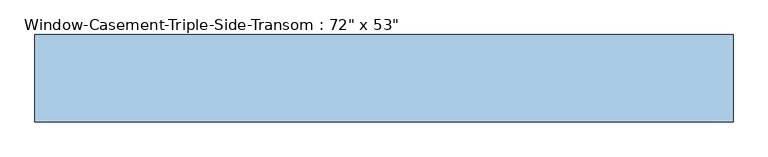
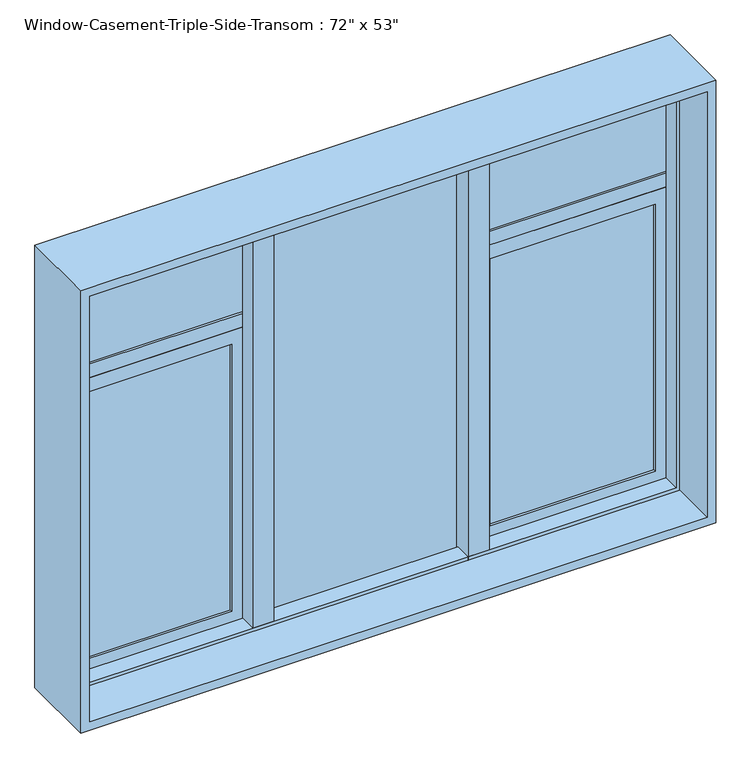
"""IFC4 building model written with IfcOpenShell, lengths in millimetres: window geometry."""

from ifc_helpers import new_model, si_unit, frame, origin, place, context, project, spatial, polyline, outline, extrude, faceted_brep, source, transform, mapped, element, save


def window_dd70d674(model_context):
    return source(origin(), model_context, "Body", "SolidModel", [
        faceted_brep([(-889.0, 73.025, 2235.2), (-889.0, 114.3, 2235.2), (889.0, 114.3, 2235.2), (889.0, 73.025, 2235.2), (-878.8796875, 22.225, 2225.0796875), (-878.8796875, 73.025, 2225.0796875), (878.8796875, 73.025, 2225.0796875), (878.8796875, 22.225, 2225.0796875), (-889.0, -114.3, 2235.2), (-889.0, 22.225, 2235.2), (889.0, 22.225, 2235.2), (889.0, -114.3, 2235.2), (-914.4, 114.3, 2260.6), (-914.4, -114.3, 2260.6), (914.4, -114.3, 2260.6), (914.4, 114.3, 2260.6), (889.0, 114.3, 939.8), (889.0, 73.025, 939.8), (878.8796875, 73.025, 949.9203125), (878.8796875, 22.225, 949.9203125), (889.0, 22.225, 939.8), (889.0, -114.3, 939.8), (914.4, -114.3, 914.4), (914.4, 114.3, 914.4), (-889.0, 114.3, 939.8), (-889.0, 73.025, 939.8), (-878.8796875, 73.025, 949.9203125), (-878.8796875, 22.225, 949.9203125), (-889.0, 22.225, 939.8), (-889.0, -114.3, 939.8), (-914.4, -114.3, 914.4), (-914.4, 114.3, 914.4)], [[[0, 1, 2, 3]], [[4, 5, 6, 7]], [[8, 9, 10, 11]], [[12, 13, 14, 15]], [[3, 2, 16, 17]], [[7, 6, 18, 19]], [[11, 10, 20, 21]], [[15, 14, 22, 23]], [[17, 16, 24, 25]], [[19, 18, 26, 27]], [[21, 20, 28, 29]], [[23, 22, 30, 31]], [[25, 24, 1, 0]], [[3, 17, 25, 0], [5, 26, 18, 6]], [[27, 26, 5, 4]], [[9, 28, 20, 10], [7, 19, 27, 4]], [[29, 28, 9, 8]], [[13, 30, 22, 14], [11, 21, 29, 8]], [[31, 30, 13, 12]], [[15, 23, 31, 12], [1, 24, 16, 2]]]),
        extrude(outline(polyline([(-279.4, 111.125), (-279.4, 22.225), (-340.3203125, 22.225), (-340.3203125, 73.025), (-330.2, 73.025), (-330.2, 111.125), (-279.4, 111.125)])), frame((0.0, 0.0, 939.8), z_axis=(0.0, 0.0, 1.0), x_axis=(1.0, 0.0, 0.0)), (0.0, 0.0, 1.0), 1295.4),
        extrude(outline(polyline([(330.2, 111.125), (330.2, 73.025), (340.3203125, 73.025), (340.3203125, 22.225), (279.4, 22.225), (279.4, 111.125), (330.2, 111.125)])), frame((0.0, 0.0, 939.8), z_axis=(0.0, 0.0, 1.0), x_axis=(1.0, 0.0, 0.0)), (0.0, 0.0, 1.0), 1295.4),
        extrude(outline(polyline([(1835.8048438, 330.2), (939.8, 330.2), (939.8, 889.0), (1835.8048438, 889.0), (1835.8048438, 330.2)]), holes=[polyline([(1793.9345313, 847.1296875), (981.6703125, 847.1296875), (981.6703125, 372.0703125), (1793.9345313, 372.0703125), (1793.9345313, 847.1296875)])]), frame((0.0, 73.025, 0.0), z_axis=(0.0, 1.0, 0.0), x_axis=(0.0, 0.0, 1.0)), (0.0, 0.0, 1.0), 31.75),
        extrude(outline(polyline([(1835.8048438, -889.0), (939.8, -889.0), (939.8, -330.2), (1835.8048438, -330.2), (1835.8048438, -889.0)]), holes=[polyline([(1793.9345313, -372.0703125), (981.6703125, -372.0703125), (981.6703125, -847.1296875), (1793.9345313, -847.1296875), (1793.9345313, -372.0703125)])]), frame((0.0, 73.025, 0.0), z_axis=(0.0, 1.0, 0.0), x_axis=(0.0, 0.0, 1.0)), (0.0, 0.0, 1.0), 31.75),
        extrude(outline(polyline([(-372.0703125, 98.425), (-372.0703125, 92.075), (-847.1296875, 92.075), (-847.1296875, 98.425), (-372.0703125, 98.425)])), frame((0.0, 0.0, 981.6703125), z_axis=(0.0, 0.0, 1.0), x_axis=(1.0, 0.0, 0.0)), (0.0, 0.0, 1.0), 812.2642188),
        extrude(outline(polyline([(-372.0703125, 85.725), (-372.0703125, 79.375), (-847.1296875, 79.375), (-847.1296875, 85.725), (-372.0703125, 85.725)])), frame((0.0, 0.0, 981.6703125), z_axis=(0.0, 0.0, 1.0), x_axis=(1.0, 0.0, 0.0)), (0.0, 0.0, 1.0), 812.2642188),
        extrude(outline(polyline([(847.1296875, 98.425), (847.1296875, 92.075), (372.0703125, 92.075), (372.0703125, 98.425), (847.1296875, 98.425)])), frame((0.0, 0.0, 981.6703125), z_axis=(0.0, 0.0, 1.0), x_axis=(1.0, 0.0, 0.0)), (0.0, 0.0, 1.0), 812.2642188),
        extrude(outline(polyline([(847.1296875, 85.725), (847.1296875, 79.375), (372.0703125, 79.375), (372.0703125, 85.725), (847.1296875, 85.725)])), frame((0.0, 0.0, 981.6703125), z_axis=(0.0, 0.0, 1.0), x_axis=(1.0, 0.0, 0.0)), (0.0, 0.0, 1.0), 812.2642188),
        extrude(outline(polyline([(889.0, 104.775), (889.0, 73.025), (330.2, 73.025), (330.2, 104.775), (889.0, 104.775)])), frame((0.0, 0.0, 1835.8048438), z_axis=(0.0, 0.0, 1.0), x_axis=(1.0, 0.0, 0.0)), (0.0, 0.0, 1.0), 41.8703125),
        extrude(outline(polyline([(279.4, 98.425), (279.4, 92.075), (-279.4, 92.075), (-279.4, 98.425), (279.4, 98.425)])), frame((0.0, 0.0, 939.8), z_axis=(0.0, 0.0, 1.0), x_axis=(1.0, 0.0, 0.0)), (0.0, 0.0, 1.0), 1295.4),
        extrude(outline(polyline([(279.4, 85.725), (279.4, 79.375), (-279.4, 79.375), (-279.4, 85.725), (279.4, 85.725)])), frame((0.0, 0.0, 939.8), z_axis=(0.0, 0.0, 1.0), x_axis=(1.0, 0.0, 0.0)), (0.0, 0.0, 1.0), 1295.4),
        extrude(outline(polyline([(-330.2, 104.775), (-330.2, 73.025), (-889.0, 73.025), (-889.0, 104.775), (-330.2, 104.775)])), frame((0.0, 0.0, 1835.8048438), z_axis=(0.0, 0.0, 1.0), x_axis=(1.0, 0.0, 0.0)), (0.0, 0.0, 1.0), 41.8703125),
        extrude(outline(polyline([(-330.2, 98.425), (-330.2, 92.075), (-889.0, 92.075), (-889.0, 98.425), (-330.2, 98.425)])), frame((0.0, 0.0, 1877.6751562), z_axis=(0.0, 0.0, 1.0), x_axis=(1.0, 0.0, 0.0)), (0.0, 0.0, 1.0), 357.5248438),
        extrude(outline(polyline([(-330.2, 85.725), (-330.2, 79.375), (-889.0, 79.375), (-889.0, 85.725), (-330.2, 85.725)])), frame((0.0, 0.0, 1877.6751562), z_axis=(0.0, 0.0, 1.0), x_axis=(1.0, 0.0, 0.0)), (0.0, 0.0, 1.0), 357.5248438),
        extrude(outline(polyline([(889.0, 98.425), (889.0, 92.075), (330.2, 92.075), (330.2, 98.425), (889.0, 98.425)])), frame((0.0, 0.0, 1877.6751562), z_axis=(0.0, 0.0, 1.0), x_axis=(1.0, 0.0, 0.0)), (0.0, 0.0, 1.0), 357.5248438),
        extrude(outline(polyline([(889.0, 85.725), (889.0, 79.375), (330.2, 79.375), (330.2, 85.725), (889.0, 85.725)])), frame((0.0, 0.0, 1877.6751562), z_axis=(0.0, 0.0, 1.0), x_axis=(1.0, 0.0, 0.0)), (0.0, 0.0, 1.0), 357.5248438),
    ])


if __name__ == "__main__":
    model = new_model("IFC4")
    model_context = context("Model", 3, world=origin())
    ifc_project = project(units=[si_unit("LENGTHUNIT", "METRE", prefix="MILLI")], contexts=[model_context])
    site = spatial("IfcSite", under=ifc_project)
    building = spatial("IfcBuilding", under=site)
    placement = place(None, origin())
    window_shape = window_dd70d674(model_context)
    element("IfcWindow", 1, ObjectType="Window-Casement-Triple-Side-Transom : 72\" x 53\"", at=placement, inside=building, context=model_context, shape_type="MappedRepresentation", body=[
        mapped(window_shape, transform((0.0, 0.0, 0.0), x_axis=(1.0, 0.0, 0.0), y_axis=(0.0, 1.0, 0.0), z_axis=(0.0, 0.0, 1.0))),
    ])
    save(model, "model.ifc")

# Revit data of these elements
# Type "Window-Casement-Triple-Side-Transom : 72\" x 53\""
#   Type Mark = "19"
#   Fire Rating = "0.5h"
#   Analytic Construction = "Double glazing - domestic"
#   Window Width = 2' - 0"
#   Window Inset [instance default] = 0' - 0 5/8"
#   Wall Thickness [instance default] = 0' - 6"
#   Visual Light Transmittance = 0.81
#   Transom Height Ratio = 0.3
#   Thermal Resistance (R) = 1.8146 (h·ft²·°F)/BTU
#   Solar Heat Gain Coefficient = 0.76
#   Rough Width = 6' - 0 1/2"
#   Rough Height = 4' - 5 1/2"
#   Open Window Height = 3' - 1.1"
#   Heat Transfer Coefficient (U) = 0.5511 BTU/(h·ft²·°F)
#   Height = 4' - 5"
#   Transom Height = 1' - 3.9"
#   Frame Gap 3 [instance default] = 0' - 1 83/128"
#   Frame Gap 2 [instance default] = 0' - 0 5/8"
#   Frame Gap 1 = 0' - 1 51/128"
#   Default Sill Height = 3' - 0"
#   Width = 6' - 0"
#   Frame Material = Metal - Aluminum
#   Glass Panel Material = Glass
#   Wall Closure = (empty or 0)
# Element 1 (IfcWindow, "Window-Casement-Triple-Side-Transom : 72\" x 53\"")
#   Wall Thickness = 0' - 9"
#   Materials on its faces: "Metal - Aluminum", "Glass"
# Materials
#   "Metal - Aluminum": class "Metal", colour RGB 247 247 247, transparency 0
#   "Glass": class "Glass", colour RGB 0 128 192, transparency 0.75, Description = "Soda Lime Glass", Cost = 0
